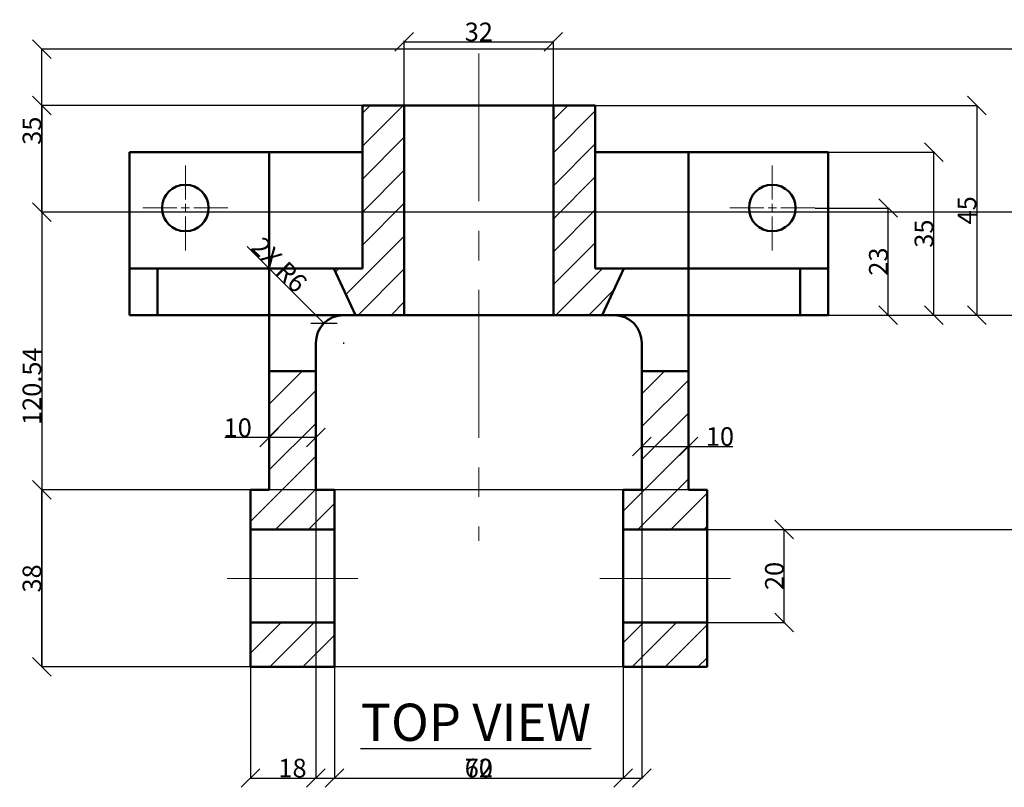
# Model space of a CAD drawing. Units: millimetres. Extents: x 113 to 503, y 39 to 409.
# Tile 1 of 3: x 120 to 332, y 39 to 204. Entities that reach past the tile are written whole.
import ezdxf

# ---------------------------------------------------------------- set-up
doc = ezdxf.new("R2010")
doc.units = ezdxf.units.MM
doc.header["$MEASUREMENT"] = 0
doc.linetypes.add('CENTER', pattern=[50.8, 31.75, -6.35, 6.35, -6.35])
for name, color, linetype, lineweight in [('M-CNTR', 1, 'CENTER', 18), ('M-DIMS', 2, 'Continuous', 25), ('M-HATC', 8, 'Continuous', 18), ('M-OUTL', 7, 'Continuous', 50), ('M-TEXT', 3, 'Continuous', 25)]:
    doc.layers.add(name, color=color, linetype=linetype, lineweight=lineweight)
doc.styles.get("Standard").update_dxf_attribs({"font": 'arial.ttf'})
doc.dimstyles.get("Standard").update_dxf_attribs({"dimtxt": 4, "dimasz": 4, "dimexe": 0.18, "dimexo": 0.0625, "dimgap": 0.09, "dimtad": 1, "dimdec": 0, "dimzin": 0, "dimdsep": 46, "dimtxsty": 'Standard', "dimblk": 'OBLIQUE', "dimcen": 0.09, "dimclre": 251, "dimadec": 0, "dimazin": 0, "dimtfac": 1, "dimtdec": 0, "dimtofl": 0, "dimtmove": 0, "dimatfit": 3, "dimfxl": 1, "dimtolj": 1, "dimtzin": 0, "dimarcsym": 0})

# ---------------------------------------------------------------- blocks, each defined once
blk = doc.blocks.new('*U22')
at = {"layer": 'M-CNTR', "color": 0, "transparency": 16777216}
for p, q in [((0, 1.8), (0, 9.12)), ((-9.12, 0), (-1.8, 0)), ((1.8, 0), (9.12, 0)), ((0, -9.12), (0, -1.8))]:
    blk.add_line(p, q, dxfattribs=at)
at = {"layer": 'M-CNTR', "color": 0, "linetype": 'Continuous', "transparency": 16777216}
for p, q in [((-0.9, 0), (0.9, 0)), ((0, -0.9), (0, 0.9))]:
    blk.add_line(p, q, dxfattribs=at)
blk = doc.blocks.new('*U23')
at = {"layer": 'M-CNTR', "color": 0, "transparency": 16777216}
for p, q in [((0, 1.8), (0, 9.12)), ((-9.12, 0), (-1.8, 0)), ((1.8, 0), (9.12, 0)), ((0, -9.12), (0, -1.8))]:
    blk.add_line(p, q, dxfattribs=at)
at = {"layer": 'M-CNTR', "color": 0, "linetype": 'Continuous', "transparency": 16777216}
for p, q in [((-0.9, 0), (0.9, 0)), ((0, -0.9), (0, 0.9))]:
    blk.add_line(p, q, dxfattribs=at)
blk = doc.blocks.new('_Oblique')
at = {"color": 0, "linetype": 'ByBlock', "lineweight": -2}
blk.add_line((-0.5, -0.5), (0.5, 0.5), dxfattribs=at)
blk = doc.blocks.new('*D24')
at = {"layer": 'Defpoints', "color": 0, "transparency": 16777216}
for p in [(234.81, 199.35), (202.81, 185.67), (234.81, 185.67)]:
    blk.add_point(p, dxfattribs=at)
at = {"layer": 'M-DIMS', "color": 0, "lineweight": -2, "transparency": 16777216}
for p, q in [((202.81, 185.74), (202.81, 199.53)), ((202.81, 199.35), (234.81, 199.35)), ((234.81, 185.74), (234.81, 199.53))]:
    blk.add_line(p, q, dxfattribs=at)
at = {"layer": 'M-DIMS', "color": 0, "lineweight": -2, "transparency": 16777216, "xscale": 4, "yscale": 4, "zscale": 4, "rotation": 180}
blk.add_blockref('_Oblique', (202.81, 199.35), dxfattribs=at)
at = {"layer": 'M-DIMS', "color": 0, "lineweight": -2, "transparency": 16777216, "xscale": 4, "yscale": 4, "zscale": 4}
blk.add_blockref('_Oblique', (234.81, 199.35), dxfattribs=at)
at = {"layer": 'M-DIMS', "color": 0, "transparency": 16777216, "insert": (218.81, 201.48), "char_height": 4, "attachment_point": 5}
blk.add_mtext('\\A1;32', dxfattribs=at)
blk = doc.blocks.new('*D25')
at = {"layer": 'Defpoints', "color": 0, "transparency": 16777216}
for p in [(290.93, 163.67), (306.71, 163.67), (293.81, 140.67)]:
    blk.add_point(p, dxfattribs=at)
at = {"layer": 'M-DIMS', "color": 0, "lineweight": -2, "transparency": 16777216}
for p, q in [((290.99, 163.67), (306.89, 163.67)), ((306.71, 140.67), (306.71, 163.67)), ((293.87, 140.67), (306.89, 140.67))]:
    blk.add_line(p, q, dxfattribs=at)
at = {"layer": 'M-DIMS', "color": 0, "lineweight": -2, "transparency": 16777216, "xscale": 4, "yscale": 4, "zscale": 4}
for p, rotation in [((306.71, 163.67), 90), ((306.71, 140.67), 270)]:
    blk.add_blockref('_Oblique', p, dxfattribs=dict(at, rotation=rotation))
at = {"layer": 'M-DIMS', "color": 0, "transparency": 16777216, "insert": (304.57, 152.17), "char_height": 4, "attachment_point": 5, "rotation": 90}
blk.add_mtext('\\A1;23', dxfattribs=at)
blk = doc.blocks.new('*D26')
at = {"layer": 'Defpoints', "color": 0, "transparency": 16777216}
for p in [(293.81, 175.67), (316.49, 175.67), (293.81, 140.67)]:
    blk.add_point(p, dxfattribs=at)
at = {"layer": 'M-DIMS', "color": 0, "lineweight": -2, "transparency": 16777216}
for p, q in [((293.87, 175.67), (316.67, 175.67)), ((316.49, 140.67), (316.49, 175.67)), ((293.87, 140.67), (316.67, 140.67))]:
    blk.add_line(p, q, dxfattribs=at)
at = {"layer": 'M-DIMS', "color": 0, "lineweight": -2, "transparency": 16777216, "xscale": 4, "yscale": 4, "zscale": 4}
for p, rotation in [((316.49, 175.67), 90), ((316.49, 140.67), 270)]:
    blk.add_blockref('_Oblique', p, dxfattribs=dict(at, rotation=rotation))
at = {"layer": 'M-DIMS', "color": 0, "transparency": 16777216, "insert": (314.36, 158.17), "char_height": 4, "attachment_point": 5, "rotation": 90}
blk.add_mtext('\\A1;35', dxfattribs=at)
blk = doc.blocks.new('*D27')
at = {"layer": 'Defpoints', "color": 0, "transparency": 16777216}
for p in [(243.81, 185.67), (293.81, 140.67), (325.71, 140.67)]:
    blk.add_point(p, dxfattribs=at)
at = {"layer": 'M-DIMS', "color": 0, "lineweight": -2, "transparency": 16777216}
for p, q in [((243.87, 185.67), (325.89, 185.67)), ((325.71, 185.67), (325.71, 140.67)), ((293.87, 140.67), (325.89, 140.67))]:
    blk.add_line(p, q, dxfattribs=at)
at = {"layer": 'M-DIMS', "color": 0, "lineweight": -2, "transparency": 16777216, "xscale": 4, "yscale": 4, "zscale": 4}
for p, rotation in [((325.71, 185.67), 90), ((325.71, 140.67), 270)]:
    blk.add_blockref('_Oblique', p, dxfattribs=dict(at, rotation=rotation))
at = {"layer": 'M-DIMS', "color": 0, "transparency": 16777216, "insert": (323.59, 163.17), "char_height": 4, "attachment_point": 5, "rotation": 90}
blk.add_mtext('\\A1;45', dxfattribs=at)
blk = doc.blocks.new('*D28')
at = {"layer": 'Defpoints', "color": 0, "transparency": 16777216}
for p in [(253.81, 113.08), (263.81, 113.08), (263.81, 112.48)]:
    blk.add_point(p, dxfattribs=at)
at = {"layer": 'M-DIMS', "color": 0, "lineweight": -2, "transparency": 16777216}
for p, q in [((253.81, 113.02), (253.81, 112.3)), ((253.81, 112.48), (263.81, 112.48)), ((263.81, 113.02), (263.81, 112.3)), ((263.81, 112.48), (273.33, 112.48))]:
    blk.add_line(p, q, dxfattribs=at)
at = {"layer": 'M-DIMS', "color": 0, "lineweight": -2, "transparency": 16777216, "xscale": 4, "yscale": 4, "zscale": 4, "rotation": 180}
blk.add_blockref('_Oblique', (253.81, 112.48), dxfattribs=at)
at = {"layer": 'M-DIMS', "color": 0, "lineweight": -2, "transparency": 16777216, "xscale": 4, "yscale": 4, "zscale": 4}
blk.add_blockref('_Oblique', (263.81, 112.48), dxfattribs=at)
at = {"layer": 'M-DIMS', "color": 0, "transparency": 16777216, "insert": (270.57, 114.61), "char_height": 4, "attachment_point": 5}
blk.add_mtext('\\A1;10', dxfattribs=at)
blk = doc.blocks.new('*D29')
at = {"layer": 'Defpoints', "color": 0, "transparency": 16777216}
for p in [(173.81, 114.97), (173.81, 114.37), (183.81, 114.97)]:
    blk.add_point(p, dxfattribs=at)
at = {"layer": 'M-DIMS', "color": 0, "lineweight": -2, "transparency": 16777216}
for p, q in [((173.81, 114.37), (164.29, 114.37)), ((173.81, 114.91), (173.81, 114.19)), ((183.81, 114.37), (173.81, 114.37)), ((183.81, 114.91), (183.81, 114.19))]:
    blk.add_line(p, q, dxfattribs=at)
at = {"layer": 'M-DIMS', "color": 0, "lineweight": -2, "transparency": 16777216, "xscale": 4, "yscale": 4, "zscale": 4, "rotation": 180}
blk.add_blockref('_Oblique', (173.81, 114.37), dxfattribs=at)
at = {"layer": 'M-DIMS', "color": 0, "lineweight": -2, "transparency": 16777216, "xscale": 4, "yscale": 4, "zscale": 4}
blk.add_blockref('_Oblique', (183.81, 114.37), dxfattribs=at)
at = {"layer": 'M-DIMS', "color": 0, "transparency": 16777216, "insert": (167.05, 116.5), "char_height": 4, "attachment_point": 5}
blk.add_mtext('\\A1;10', dxfattribs=at)
blk = doc.blocks.new('*D30')
at = {"layer": 'Defpoints', "color": 0, "transparency": 16777216}
for p in [(267.81, 94.67), (284.39, 94.67), (267.81, 74.67)]:
    blk.add_point(p, dxfattribs=at)
at = {"layer": 'M-DIMS', "color": 0, "lineweight": -2, "transparency": 16777216}
for p, q in [((267.87, 94.67), (284.57, 94.67)), ((284.39, 74.67), (284.39, 94.67)), ((267.87, 74.67), (284.57, 74.67))]:
    blk.add_line(p, q, dxfattribs=at)
at = {"layer": 'M-DIMS', "color": 0, "lineweight": -2, "transparency": 16777216, "xscale": 4, "yscale": 4, "zscale": 4}
for p, rotation in [((284.39, 94.67), 90), ((284.39, 74.67), 270)]:
    blk.add_blockref('_Oblique', p, dxfattribs=dict(at, rotation=rotation))
at = {"layer": 'M-DIMS', "color": 0, "transparency": 16777216, "insert": (282.26, 84.67), "char_height": 4, "attachment_point": 5, "rotation": 90}
blk.add_mtext('\\A1;20', dxfattribs=at)
blk = doc.blocks.new('*D37')
at = {"layer": 'Defpoints', "color": 0, "transparency": 16777216}
for p in [(125.01, 103.14), (267.81, 103.14), (267.81, 65.14)]:
    blk.add_point(p, dxfattribs=at)
at = {"layer": 'M-DIMS', "color": 251, "lineweight": -2, "transparency": 16777216}
for p, q in [((267.75, 103.14), (124.83, 103.14)), ((267.75, 65.14), (124.83, 65.14))]:
    blk.add_line(p, q, dxfattribs=at)
at = {"layer": 'M-DIMS', "color": 0, "lineweight": -2, "transparency": 16777216}
blk.add_line((125.01, 65.14), (125.01, 103.14), dxfattribs=at)
at = {"layer": 'M-DIMS', "color": 0, "lineweight": -2, "transparency": 16777216, "xscale": 4, "yscale": 4, "zscale": 4}
for p, rotation in [((125.01, 103.14), 90), ((125.01, 65.14), 270)]:
    blk.add_blockref('_Oblique', p, dxfattribs=dict(at, rotation=rotation))
at = {"layer": 'M-DIMS', "color": 0, "transparency": 16777216, "insert": (122.88, 84.14), "char_height": 4, "attachment_point": 5, "rotation": 90}
blk.add_mtext('\\A1;38', dxfattribs=at)
blk = doc.blocks.new('*D38')
at = {"layer": 'Defpoints', "color": 0, "transparency": 16777216}
for p in [(293.81, 140.67), (501.29, 140.67), (267.81, 94.67)]:
    blk.add_point(p, dxfattribs=at)
at = {"layer": 'M-DIMS', "color": 251, "lineweight": -2, "transparency": 16777216}
for p, q in [((293.87, 140.67), (501.47, 140.67)), ((267.87, 94.67), (501.47, 94.67))]:
    blk.add_line(p, q, dxfattribs=at)
at = {"layer": 'M-DIMS', "color": 0, "lineweight": -2, "transparency": 16777216}
blk.add_line((501.29, 94.67), (501.29, 140.67), dxfattribs=at)
at = {"layer": 'M-DIMS', "color": 0, "lineweight": -2, "transparency": 16777216, "xscale": 4, "yscale": 4, "zscale": 4}
for p, rotation in [((501.29, 140.67), 90), ((501.29, 94.67), 270)]:
    blk.add_blockref('_Oblique', p, dxfattribs=dict(at, rotation=rotation))
at = {"layer": 'M-DIMS', "color": 0, "transparency": 16777216, "insert": (499.16, 117.67), "char_height": 4, "attachment_point": 5, "rotation": 90}
blk.add_mtext('\\A1;46', dxfattribs=at)
blk = doc.blocks.new('*D39')
at = {"layer": 'Defpoints', "color": 0, "transparency": 16777216}
for p in [(169.81, 65.14), (187.81, 65.14), (187.81, 41.29)]:
    blk.add_point(p, dxfattribs=at)
at = {"layer": 'M-DIMS', "color": 251, "lineweight": -2, "transparency": 16777216}
for p, q in [((169.81, 65.08), (169.81, 41.11)), ((187.81, 65.08), (187.81, 41.11))]:
    blk.add_line(p, q, dxfattribs=at)
at = {"layer": 'M-DIMS', "color": 0, "lineweight": -2, "transparency": 16777216}
blk.add_line((169.81, 41.29), (187.81, 41.29), dxfattribs=at)
at = {"layer": 'M-DIMS', "color": 0, "lineweight": -2, "transparency": 16777216, "xscale": 4, "yscale": 4, "zscale": 4, "rotation": 180}
blk.add_blockref('_Oblique', (169.81, 41.29), dxfattribs=at)
at = {"layer": 'M-DIMS', "color": 0, "lineweight": -2, "transparency": 16777216, "xscale": 4, "yscale": 4, "zscale": 4}
blk.add_blockref('_Oblique', (187.81, 41.29), dxfattribs=at)
at = {"layer": 'M-DIMS', "color": 0, "transparency": 16777216, "insert": (178.81, 43.42), "char_height": 4, "attachment_point": 5}
blk.add_mtext('\\A1;18', dxfattribs=at)
blk = doc.blocks.new('*D40')
at = {"layer": 'Defpoints', "color": 0, "transparency": 16777216}
for p in [(187.81, 65.14), (249.81, 65.14), (249.81, 41.29)]:
    blk.add_point(p, dxfattribs=at)
at = {"layer": 'M-DIMS', "color": 251, "lineweight": -2, "transparency": 16777216}
for p, q in [((187.81, 65.08), (187.81, 41.11)), ((249.81, 65.08), (249.81, 41.11))]:
    blk.add_line(p, q, dxfattribs=at)
at = {"layer": 'M-DIMS', "color": 0, "lineweight": -2, "transparency": 16777216}
blk.add_line((187.81, 41.29), (249.81, 41.29), dxfattribs=at)
at = {"layer": 'M-DIMS', "color": 0, "lineweight": -2, "transparency": 16777216, "xscale": 4, "yscale": 4, "zscale": 4, "rotation": 180}
blk.add_blockref('_Oblique', (187.81, 41.29), dxfattribs=at)
at = {"layer": 'M-DIMS', "color": 0, "lineweight": -2, "transparency": 16777216, "xscale": 4, "yscale": 4, "zscale": 4}
blk.add_blockref('_Oblique', (249.81, 41.29), dxfattribs=at)
at = {"layer": 'M-DIMS', "color": 0, "transparency": 16777216, "insert": (218.81, 43.42), "char_height": 4, "attachment_point": 5}
blk.add_mtext('\\A1;62', dxfattribs=at)
blk = doc.blocks.new('*D41')
at = {"layer": 'Defpoints', "color": 0, "transparency": 16777216}
for p in [(183.81, 103.14), (253.81, 103.14), (253.81, 41.29)]:
    blk.add_point(p, dxfattribs=at)
at = {"layer": 'M-DIMS', "color": 251, "lineweight": -2, "transparency": 16777216}
for p, q in [((183.81, 103.08), (183.81, 41.11)), ((253.81, 103.08), (253.81, 41.11))]:
    blk.add_line(p, q, dxfattribs=at)
at = {"layer": 'M-DIMS', "color": 0, "lineweight": -2, "transparency": 16777216}
blk.add_line((183.81, 41.29), (253.81, 41.29), dxfattribs=at)
at = {"layer": 'M-DIMS', "color": 0, "lineweight": -2, "transparency": 16777216, "xscale": 4, "yscale": 4, "zscale": 4, "rotation": 180}
blk.add_blockref('_Oblique', (183.81, 41.29), dxfattribs=at)
at = {"layer": 'M-DIMS', "color": 0, "lineweight": -2, "transparency": 16777216, "xscale": 4, "yscale": 4, "zscale": 4}
blk.add_blockref('_Oblique', (253.81, 41.29), dxfattribs=at)
at = {"layer": 'M-DIMS', "color": 0, "transparency": 16777216, "insert": (218.81, 43.42), "char_height": 4, "attachment_point": 5}
blk.add_mtext('\\A1;70', dxfattribs=at)
blk = doc.blocks.new('*D42')
at = {"layer": 'Defpoints', "color": 0, "transparency": 16777216}
for p in [(193.81, 185.67), (125.01, 65.14), (169.81, 65.14)]:
    blk.add_point(p, dxfattribs=at)
at = {"layer": 'M-DIMS', "color": 251, "lineweight": -2, "transparency": 16777216}
for p, q in [((193.75, 185.67), (124.83, 185.67)), ((169.75, 65.14), (124.83, 65.14))]:
    blk.add_line(p, q, dxfattribs=at)
at = {"layer": 'M-DIMS', "color": 0, "lineweight": -2, "transparency": 16777216}
blk.add_line((125.01, 185.67), (125.01, 65.14), dxfattribs=at)
at = {"layer": 'M-DIMS', "color": 0, "lineweight": -2, "transparency": 16777216, "xscale": 4, "yscale": 4, "zscale": 4}
for p, rotation in [((125.01, 185.67), 90), ((125.01, 65.14), 270)]:
    blk.add_blockref('_Oblique', p, dxfattribs=dict(at, rotation=rotation))
at = {"layer": 'M-DIMS', "color": 0, "transparency": 16777216, "insert": (122.88, 125.41), "char_height": 4, "attachment_point": 5, "rotation": 90}
blk.add_mtext('\\A1;120.54', dxfattribs=at)
blk = doc.blocks.new('*D47')
at = {"layer": 'Defpoints', "color": 0, "transparency": 16777216}
for p in [(125.01, 197.77), (397.49, 197.77), (397.49, 162.77)]:
    blk.add_point(p, dxfattribs=at)
at = {"layer": 'M-DIMS', "color": 251, "lineweight": -2, "transparency": 16777216}
for p, q in [((397.43, 197.77), (124.83, 197.77)), ((397.43, 162.77), (124.83, 162.77))]:
    blk.add_line(p, q, dxfattribs=at)
at = {"layer": 'M-DIMS', "color": 0, "lineweight": -2, "transparency": 16777216}
blk.add_line((125.01, 162.77), (125.01, 197.77), dxfattribs=at)
at = {"layer": 'M-DIMS', "color": 0, "lineweight": -2, "transparency": 16777216, "xscale": 4, "yscale": 4, "zscale": 4}
for p, rotation in [((125.01, 197.77), 90), ((125.01, 162.77), 270)]:
    blk.add_blockref('_Oblique', p, dxfattribs=dict(at, rotation=rotation))
at = {"layer": 'M-DIMS', "color": 0, "transparency": 16777216, "insert": (122.88, 180.27), "char_height": 4, "attachment_point": 5, "rotation": 90}
blk.add_mtext('\\A1;35', dxfattribs=at)
blk = doc.blocks.new('*D54')
at = {"layer": 'Defpoints', "color": 0, "transparency": 16777216}
for p in [(185.57, 138.92), (189.81, 134.67)]:
    blk.add_point(p, dxfattribs=at)
at = {"layer": 'M-DIMS', "color": 0, "lineweight": -2, "transparency": 16777216}
blk.add_line((169.1, 155.39), (185.57, 138.92), dxfattribs=at)
at = {"layer": 'M-DIMS', "color": 251, "lineweight": -2, "transparency": 16777216}
for p, q in [((189.72, 134.67), (189.9, 134.67)), ((189.81, 134.58), (189.81, 134.76))]:
    blk.add_line(p, q, dxfattribs=at)
at = {"layer": 'M-DIMS', "color": 0, "lineweight": -2, "transparency": 16777216, "xscale": 4, "yscale": 4, "zscale": 4, "rotation": 314.998237630734}
blk.add_blockref('_Oblique', (185.57, 138.92), dxfattribs=at)
at = {"layer": 'M-DIMS', "color": 0, "transparency": 16777216, "insert": (176.01, 151.49), "char_height": 4, "attachment_point": 5, "rotation": 314.9982}
blk.add_mtext('\\A1;2X R6', dxfattribs=at)

msp = doc.modelspace()

# ---------------------------------------------------------------- hatches: boundary and pattern name
at = {"layer": 'M-HATC'}
h = msp.add_hatch(dxfattribs=at)
h.set_pattern_fill('ANSI31', color=256, scale=40)
h.set_pattern_definition([(45, (0, 223.543), (-3.53553, 3.53553), [])])
h.paths.add_polyline_path([(202.81, 185.675), (193.81, 185.675), (193.81, 150.675), (187.669, 150.675), (192.311, 140.675), (202.81, 140.675)])
h.paths.add_polyline_path([(234.81, 140.675), (245.309, 140.675), (249.952, 150.675), (243.81, 150.675), (243.81, 185.675), (234.81, 185.675)])
h.paths.add_polyline_path([(263.81, 128.67), (253.81, 128.67), (253.81, 103.139), (249.81, 103.139), (249.81, 94.675), (267.81, 94.675), (267.81, 103.139), (263.81, 103.139)])
h.paths.add_polyline_path([(173.81, 103.139), (169.81, 103.139), (169.81, 94.675), (187.81, 94.675), (187.81, 103.139), (183.81, 103.139), (183.81, 128.67), (173.81, 128.67)])
h.paths.add_polyline_path([(187.81, 65.139), (187.81, 74.675), (169.81, 74.675), (169.81, 65.139)])
h.paths.add_polyline_path([(249.81, 74.675), (249.81, 65.139), (267.81, 65.139), (267.81, 74.675)])

# ---------------------------------------------------------------- linework, layer by layer
at = {"layer": 'M-CNTR'}
for p, q in [((218.81, 196.88), (218.81, 92.191)), ((192.81, 84.139), (164.81, 84.139)), ((272.81, 84.139), (244.81, 84.139))]:
    msp.add_line(p, q, dxfattribs=at)
at = {"layer": 'M-OUTL'}
for p, q in [((193.81, 185.675), (193.81, 150.675)), ((193.81, 185.675), (243.81, 185.675)), ((202.81, 185.675), (202.81, 140.675)), ((234.81, 185.675), (234.81, 140.675)), ((243.81, 185.675), (243.81, 150.675)), ((143.81, 175.675), (193.81, 175.675)), ((143.81, 150.675), (143.81, 175.675)), ((173.81, 175.675), (173.81, 103.139)), ((243.81, 175.675), (293.81, 175.675)), ((263.81, 175.675), (263.81, 103.139)), ((293.81, 175.675), (293.81, 150.675)), ((143.81, 150.675), (193.81, 150.675)), ((143.81, 140.675), (143.81, 150.675)), ((149.81, 150.675), (149.81, 140.675)), ((187.669, 150.675), (192.311, 140.675)), ((243.81, 150.675), (293.81, 150.675)), ((249.952, 150.675), (245.309, 140.675)), ((287.81, 140.675), (287.81, 150.675)), ((293.81, 150.675), (293.81, 140.675)), ((143.81, 140.675), (293.81, 140.675)), ((183.81, 134.675), (183.81, 103.139)), ((253.81, 134.675), (253.81, 103.139)), ((173.81, 128.67), (183.81, 128.67)), ((253.81, 128.67), (263.81, 128.67)), ((169.81, 103.139), (173.81, 103.139)), ((169.81, 103.139), (169.81, 65.139)), ((183.81, 103.139), (187.81, 103.139)), ((187.81, 103.139), (187.81, 65.139)), ((253.81, 103.139), (249.81, 103.139)), ((249.81, 103.139), (249.81, 65.139)), ((263.81, 103.139), (267.81, 103.139)), ((267.81, 103.139), (267.81, 65.139)), ((187.81, 94.675), (169.81, 94.675)), ((267.81, 94.675), (249.81, 94.675)), ((187.81, 74.675), (169.81, 74.675)), ((267.81, 74.675), (249.81, 74.675)), ((169.81, 65.139), (187.81, 65.139)), ((249.81, 65.139), (267.81, 65.139))]:
    msp.add_line(p, q, dxfattribs=at)
for centre in [(155.81, 163.675), (281.81, 163.675)]:
    msp.add_circle(centre, 5, dxfattribs=at)
for centre, start, end in [((189.81, 134.675), 90, 180), ((247.81, 134.675), 0, 90)]:
    msp.add_arc(centre, 6, start, end, dxfattribs=at)

# ---------------------------------------------------------------- block references
at = {"layer": 'M-CNTR'}
for name, p in [('*U22', (155.81, 163.675)), ('*U23', (281.81, 163.675))]:
    msp.add_blockref(name, p, dxfattribs=at)

# ---------------------------------------------------------------- texts
at = {"layer": 'M-TEXT', "ltscale": 5, "insert": (193.436, 57.257), "char_height": 8, "attachment_point": 1}
msp.add_mtext_dynamic_manual_height_columns('{\\LTOP VIEW}', width=109.02237, gutter_width=1, heights=[0], dxfattribs=at)

# ---------------------------------------------------------------- dimensions: what is measured, and where the dimension line sits
at = {"layer": 'M-DIMS'}
for base, p1, p2, override, picture, middle in [((234.81, 199.346), (202.81, 185.675), (234.81, 185.675), {"dimclrd": 0, "dimclre": 0, "dimclrt": 0}, '*D24', (218.81, 201.48)), ((253.81, 41.292), (183.81, 103.139), (253.81, 103.139), {"dimdec": 0, "dimlfac": 1, "dimrnd": 0, "dimzin": 0, "dimdsep": 46, "dimlunit": 2}, '*D41', (218.81, 43.425)), ((187.81, 41.292), (169.81, 65.139), (187.81, 65.139), {"dimdec": 0, "dimlfac": 1, "dimrnd": 0, "dimzin": 0, "dimdsep": 46, "dimlunit": 2}, '*D39', (178.81, 43.425)), ((249.81, 41.292), (187.81, 65.139), (249.81, 65.139), {"dimdec": 0, "dimlfac": 1, "dimrnd": 0, "dimzin": 0, "dimdsep": 46, "dimlunit": 2}, '*D40', (218.81, 43.425))]:
    dim = msp.add_linear_dim(base=base, p1=p1, p2=p2, dimstyle='Standard', override=override, dxfattribs=at)
    dim.commit()
    dim.dimension.update_dxf_attribs({"geometry": picture, "text_midpoint": middle})
for base, p1, p2, override, picture, middle in [((125.01, 197.771), (397.495, 162.771), (397.495, 197.771), {"dimdec": 0, "dimlfac": 1, "dimrnd": 0, "dimzin": 0, "dimdsep": 46, "dimlunit": 2}, '*D47', (122.877, 180.271)), ((125.01, 65.139), (193.81, 185.675), (169.81, 65.139), {"dimdec": 2, "dimlfac": 1, "dimrnd": 0, "dimzin": 0, "dimdsep": 46, "dimlunit": 2}, '*D42', (122.878, 125.407)), ((325.712, 140.675), (243.81, 185.675), (293.81, 140.675), {"dimclrd": 0, "dimclre": 0, "dimclrt": 0}, '*D27', (323.588, 163.175)), ((316.493, 175.675), (293.81, 140.675), (293.81, 175.675), {"dimclrd": 0, "dimclre": 0, "dimclrt": 0}, '*D26', (314.359, 158.175)), ((306.707, 163.675), (293.81, 140.675), (290.93, 163.675), {"dimclrd": 0, "dimclre": 0, "dimclrt": 0}, '*D25', (304.573, 152.175)), ((501.295, 140.675), (267.81, 94.675), (293.81, 140.675), {"dimdec": 0, "dimlfac": 1, "dimrnd": 0, "dimzin": 0, "dimdsep": 46, "dimlunit": 2}, '*D38', (499.162, 117.675)), ((125.01, 103.139), (267.81, 65.139), (267.81, 103.139), {"dimdec": 0, "dimlfac": 1, "dimrnd": 0, "dimzin": 0, "dimdsep": 46, "dimlunit": 2}, '*D37', (122.877, 84.139)), ((284.389, 94.675), (267.81, 74.675), (267.81, 94.675), {"dimclrd": 0, "dimclre": 0, "dimclrt": 0}, '*D30', (282.256, 84.675))]:
    dim = msp.add_linear_dim(base=base, p1=p1, p2=p2, angle=90, dimstyle='Standard', override=override, dxfattribs=at)
    dim.commit()
    dim.dimension.update_dxf_attribs({"geometry": picture, "text_midpoint": middle})
dim = msp.add_radius_dim(center=(189.81, 134.675), mpoint=(185.568, 138.917), text='2X <>', dimstyle='Standard', override={"dimdec": 0, "dimlfac": 1, "dimrnd": 0, "dimzin": 0, "dimdsep": 46, "dimlunit": 2}, dxfattribs=at)
dim.commit()
dim.dimension.update_dxf_attribs({"geometry": '*D54', "text_midpoint": (176.013, 151.488)})
dim = msp.add_linear_dim(base=(173.81, 114.368), p1=(183.81, 114.974), p2=(173.81, 114.974), angle=180, dimstyle='Standard', override={"dimclrd": 0, "dimclre": 0, "dimclrt": 0}, dxfattribs=at)
dim.commit()
dim.dimension.update_dxf_attribs({"geometry": '*D29', "text_midpoint": (167.05, 114.368), "dimtype": 160})
dim = msp.add_linear_dim(base=(263.81, 112.476), p1=(253.81, 113.082), p2=(263.81, 113.082), dimstyle='Standard', override={"dimclrd": 0, "dimclre": 0, "dimclrt": 0}, dxfattribs=at)
dim.commit()
dim.dimension.update_dxf_attribs({"geometry": '*D28', "text_midpoint": (270.57, 112.476), "dimtype": 160})

doc.saveas('drawing.dxf')
